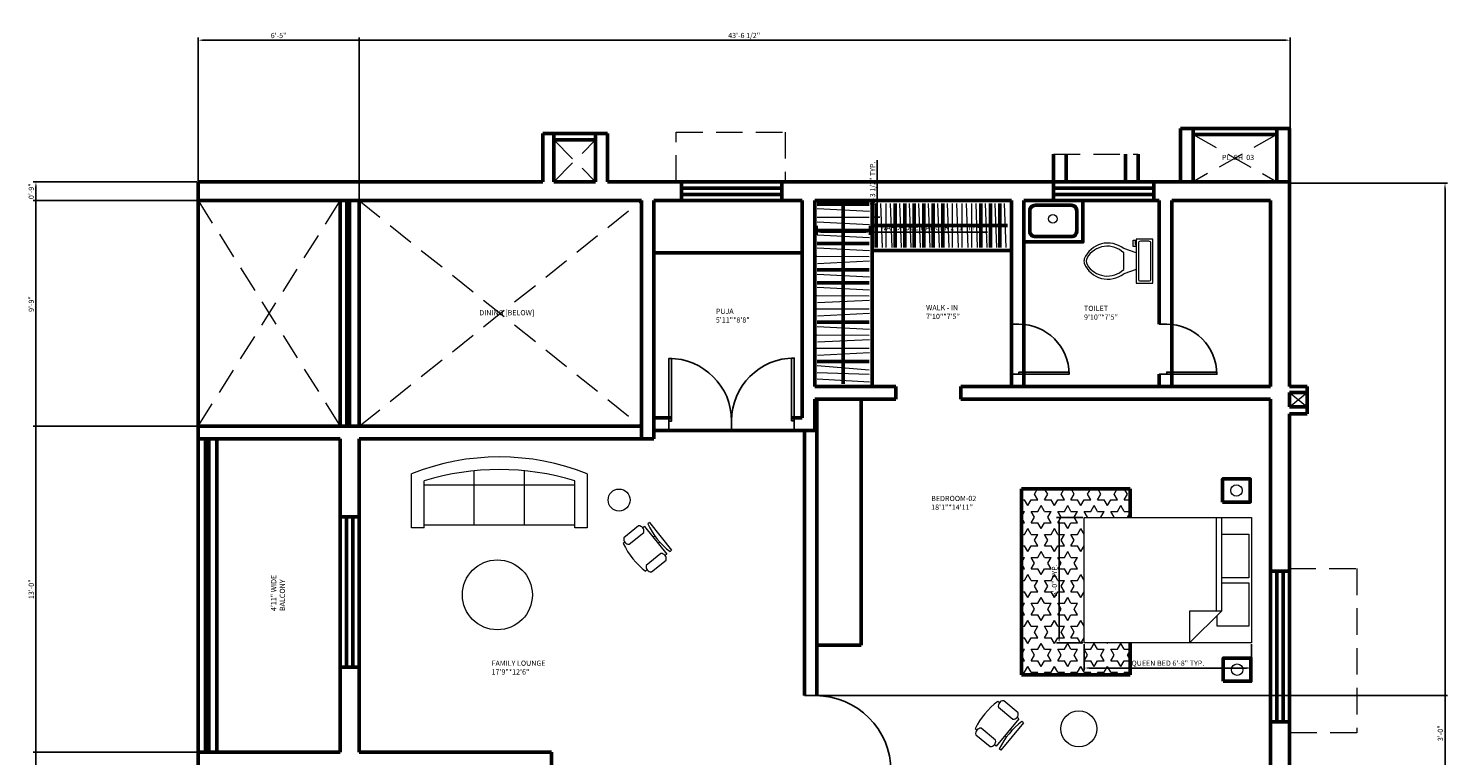
# Model space of a CAD drawing. Units: inches. Extents: x 5312 to 23584, y 2846 to 7447.
# Tile 6 of 12: x 9893 to 10572, y 3551 to 3899. Entities that reach past the tile are written whole.
import ezdxf

# ---------------------------------------------------------------- set-up
doc = ezdxf.new("R2010")
doc.units = ezdxf.units.IN
doc.linetypes.add('DASHED', pattern=[19.05, 12.7, -6.35])
for name, color, linetype, lineweight in [('A-ANNO-DIMS', 2, 'Continuous', 18), ('A-ANNO-TEXT', 3, 'Continuous', 18), ('A-AREA-IDEN', 7, 'Continuous', 18), ('A-DOOR', 4, 'Continuous', 25), ('A-FLOR-FIXT', 9, 'Continuous', 18), ('A-FLOR-OVHD', 8, 'DASHED', 18), ('A-FLOR-PATT', 252, 'Continuous', 13), ('A-FURN', 8, 'Continuous', 18), ('A-WALL', 7, 'Continuous', 50)]:
    doc.layers.add(name, color=color, linetype=linetype, lineweight=lineweight)
doc.styles.get("Standard").update_dxf_attribs({"font": 'arial.ttf'})
doc.dimstyles.new('ISO-25', dxfattribs={"dimtxt": 2.5, "dimasz": 2.5, "dimexe": 1.25, "dimexo": 0.625, "dimtad": 1, "dimlunit": 3, "dimtxsty": 'Standard', "dimcen": 2.5, "dimadec": 0, "dimazin": 0, "dimtfac": 1, "dimtmove": 0, "dimatfit": 3, "dimfxl": 1, "dimarcsym": 0})

# ---------------------------------------------------------------- blocks, each defined once
blk = doc.blocks.new('*U2')
for p, q in [((0, 0), (0, -6)), ((40, 0), (40, -6))]:
    blk.add_line(p, q)
blk.add_lwpolyline([(0, 0), (0, 40), (1.75, 40), (1.75, 0)], close=True)
blk.add_arc((0, 0), 40, 0, 90)
blk = doc.blocks.new('Sofa - Roundback 7 ft.')
for p, q in [((-12.00002, -32.4421), (-12.00003, -6.5971)), ((11.99997, -32.4421), (11.99998, -6.5971)), ((-36.000027, -34), (-36.000027, -11.4696)), ((-35.999844, -13.3819), (35.9998, -13.3819)), ((35.99998, -34), (35.99998, -11.4696)), ((-36.000027, -32.4421), (35.99998, -32.4421))]:
    blk.add_line(p, q)
for points in [[(-36.000027, -34), (-42.000027, -34), (-42.000027, -8)], [(41.99998, -8), (41.99998, -34), (35.99998, -34)]]:
    blk.add_lwpolyline(points)
for centre, radius, start, end in [((0, -114.25), 114.25, 68.43141, 111.5686), ((-0.00001, -127.1968), 121.1968, 72.72033, 107.2797)]:
    blk.add_arc(centre, radius, start, end)
blk = doc.blocks.new('Chair - Desk')
for p, q in [((-8.5, 0), (-8.5, -1)), ((-8.5, 0), (8.5, 0)), ((8.5, 0), (8.5, -1)), ((-10.5, -5), (-10.5, -14)), ((-8.5, -3), (-8.5, -4)), ((-8.5, -3), (8.5, -3)), ((-6.5, -14), (-6.5, -5)), ((-2, -3), (-2, -1.9355)), ((2, -1.9576), (2, -3)), ((6.5, -5), (6.5, -14)), ((8.5, -3), (8.5, -4)), ((10.5, -14), (10.5, -5)), ((-8.5, -15), (-8.5, -16)), ((8.5, -15), (8.5, -16))]:
    blk.add_line(p, q)
for centre, radius, start, end in [((-8.5, -6.5), 2.5, 36.8699, 143.1301), ((0, 34.625), 36.625, 256.5803, 283.4197), ((8.5, -6.5), 2.5, 36.8699, 143.1301), ((-8.5, -12.5), 2.5, 216.8699, 323.1301), ((0, 19.625), 36.625, 256.5803, 283.4197), ((8.5, -12.5), 2.5, 216.8699, 323.1301)]:
    blk.add_arc(centre, radius, start, end)
blk = doc.blocks.new('Toilet - top')
for p, q in [((9.5, -6), (9.5, -2)), ((-10, -8.5), (-8, -8.5)), ((-10, -9.5), (-10, -8.5)), ((-7, -9.5), (-10, -9.5)), ((-8, -8.5), (-8, -8)), ((-7, -8), (-7, -9.5)), ((-4, -8), (-6, -14)), ((4, -8), (6, -14)), ((4, -14), (-4, -14))]:
    blk.add_line(p, q)
blk.add_lwpolyline([(10.5, -8), (10.5, 0), (-10.5, 0), (-10.5, -8)], close=True)
for points in [[(-9.5, -2), (-9.5, -6)], [(8.5, -1), (-8.5, -1)], [(-8.5, -7), (8.5, -7)]]:
    blk.add_lwpolyline(points)
for centre, radius, start, end in [((-8.62, -1.88), 0.884, 81.8699, 188.1301), ((-8.62, -6.12), 0.884, 171.8699, 278.1301), ((8.62, -1.88), 0.884, 351.8699, 98.1301), ((8.62, -6.12), 0.884, 261.8699, 8.1301), ((3.52, -21.58), 12.17, 141.46911, 247.97143), ((4.2, -21.82), 11.33, 136.36773, 238.94682), ((-3.52, -21.58), 12.17, 292.02843, 38.53071), ((-4.2, -21.82), 11.33, 301.05301, 43.63209), ((0, -27.88), 4, 245.73182, 294.26817), ((0, -29), 4, 254.86053, 285.13947)]:
    blk.add_arc(centre, radius, start, end)
blk = doc.blocks.new('Bed - Queen')
for p, q in [((0, -80.00003), (0, 0)), ((0, 0), (59.99999, 0)), ((59.99999, 0), (59.99999, -80.00003)), ((7.99999, -1.2), (28.79998, -1.2)), ((7.99999, -14.4), (7.99999, -1.2)), ((28.79998, -1.2), (28.79998, -14.4)), ((31.19999, -1.2), (51.99999, -1.2)), ((31.19999, -14.4), (31.19999, -1.2)), ((51.99999, -1.2), (51.99999, -16.4)), ((0, -14.4), (44.8, -14.4)), ((44.8, -16.8), (0, -16.8)), ((59.99999, -29.6), (44.8, -14.4)), ((44.8, -14.4), (44.8, -29.6)), ((51.99999, -16.4), (46.79936, -16.4)), ((44.8, -29.6), (59.99999, -29.6)), ((59.99999, -80.00003), (0, -80.00003))]:
    blk.add_line(p, q)
blk = doc.blocks.new('WARDROBE-HANGER')
for p, q in [((0, 3.4), (24.8, 3.4)), ((0, 1.32), (24.99, 0))]:
    blk.add_line(p, q)
blk = doc.blocks.new('WARDROBE-HANGER-B')
for p, q in [((0, 21.08), (0.79, 0)), ((2.48, 21.08), (2.48, 0))]:
    blk.add_line(p, q)
blk = doc.blocks.new('*D25')
at = {"layer": 'A-ANNO-DIMS', "color": 0, "lineweight": -2, "transparency": 16777216}
for p, q in [((10398.36, 3604.72), (10398.36, 3592.09)), ((10478.36, 3604.72), (10478.36, 3592.09)), ((10400.86, 3593.34), (10475.86, 3593.34))]:
    blk.add_line(p, q, dxfattribs=at)
at = {"layer": 'A-ANNO-DIMS', "color": 0, "transparency": 16777216}
for points in [[(10400.86, 3593.76), (10400.86, 3592.92), (10398.36, 3593.34)], [(10475.86, 3593.76), (10475.86, 3592.92), (10478.36, 3593.34)]]:
    blk.add_solid(points, dxfattribs=at)
at = {"layer": 'DEFPOINTS', "color": 0, "transparency": 16777216}
for p in [(10398.36, 3605.34), (10478.36, 3605.34), (10478.36, 3593.34)]:
    blk.add_point(p, dxfattribs=at)
at = {"layer": 'A-ANNO-DIMS', "color": 0, "transparency": 16777216, "insert": (10438.36, 3595.33), "char_height": 2.5, "attachment_point": 5}
blk.add_mtext('QUEEN BED 6\'-8" TYP.', dxfattribs=at)
blk = doc.blocks.new('*D26')
at = {"layer": 'A-ANNO-DIMS', "color": 0, "lineweight": -2, "transparency": 16777216}
for p, q in [((10397.74, 3665.34), (10385.11, 3665.34)), ((10386.36, 3662.84), (10386.36, 3607.84)), ((10397.74, 3605.34), (10385.11, 3605.34))]:
    blk.add_line(p, q, dxfattribs=at)
at = {"layer": 'A-ANNO-DIMS', "color": 0, "transparency": 16777216}
for points in [[(10385.95, 3662.84), (10386.78, 3662.84), (10386.36, 3665.34)], [(10385.95, 3607.84), (10386.78, 3607.84), (10386.36, 3605.34)]]:
    blk.add_solid(points, dxfattribs=at)
at = {"layer": 'DEFPOINTS', "color": 0, "transparency": 16777216}
for p in [(10398.36, 3665.34), (10386.36, 3605.34), (10398.36, 3605.34)]:
    blk.add_point(p, dxfattribs=at)
at = {"layer": 'A-ANNO-DIMS', "color": 0, "transparency": 16777216, "insert": (10384.46, 3635.34), "char_height": 2.5, "attachment_point": 5, "rotation": 90}
blk.add_mtext('5\'-0" TYP.', dxfattribs=at)
blk = doc.blocks.new('*D35')
at = {"layer": 'A-ANNO-DIMS', "color": 0, "lineweight": -2, "transparency": 16777216}
for p, q in [((10270.63, 3805.02), (10270.63, 3800.65)), ((10273.13, 3801.9), (10293.12, 3801.9)), ((10295.62, 3805.02), (10295.62, 3800.65)), ((10295.62, 3801.9), (10352.16, 3801.9))]:
    blk.add_line(p, q, dxfattribs=at)
at = {"layer": 'A-ANNO-DIMS', "color": 0, "transparency": 16777216}
for points in [[(10273.13, 3802.31), (10273.13, 3801.48), (10270.63, 3801.9)], [(10293.12, 3802.31), (10293.12, 3801.48), (10295.62, 3801.9)]]:
    blk.add_solid(points, dxfattribs=at)
at = {"layer": 'DEFPOINTS', "color": 0, "transparency": 16777216}
for p in [(10270.63, 3805.65), (10295.62, 3805.65), (10295.62, 3801.9)]:
    blk.add_point(p, dxfattribs=at)
at = {"layer": 'A-ANNO-DIMS', "color": 0, "transparency": 16777216, "insert": (10325.14, 3803.82), "char_height": 2.5, "attachment_point": 5}
blk.add_mtext('WARDROBE HANGER 2\'-1" TYP.', dxfattribs=at)
blk = doc.blocks.new('*D36')
at = {"layer": 'A-ANNO-DIMS', "color": 0, "lineweight": -2, "transparency": 16777216}
for p, q in [((10299.37, 3811.55), (10299.37, 3836.36)), ((10296.25, 3809.05), (10300.62, 3809.05)), ((10299.37, 3805.65), (10299.37, 3809.05)), ((10296.25, 3805.65), (10300.62, 3805.65)), ((10299.37, 3803.15), (10299.37, 3800.65))]:
    blk.add_line(p, q, dxfattribs=at)
at = {"layer": 'A-ANNO-DIMS', "color": 0, "transparency": 16777216}
for points in [[(10298.95, 3811.55), (10299.79, 3811.55), (10299.37, 3809.05)], [(10298.95, 3803.15), (10299.79, 3803.15), (10299.37, 3805.65)]]:
    blk.add_solid(points, dxfattribs=at)
at = {"layer": 'DEFPOINTS', "color": 0, "transparency": 16777216}
for p in [(10295.62, 3809.05), (10299.37, 3809.05), (10295.62, 3805.65)]:
    blk.add_point(p, dxfattribs=at)
at = {"layer": 'A-ANNO-DIMS', "color": 0, "transparency": 16777216, "insert": (10297.45, 3825.21), "char_height": 2.5, "attachment_point": 5, "rotation": 90}
blk.add_mtext('0\'-3 1/2" TYP.', dxfattribs=at)
blk = doc.blocks.new('*D71')
at = {"layer": 'A-ANNO-DIMS', "color": 0, "lineweight": -2, "transparency": 16777216}
for p, q in [((9974.51, 3826.67), (9974.51, 3895.08)), ((9977.01, 3893.83), (10494.36, 3893.83)), ((10496.86, 3826), (10496.86, 3895.08))]:
    blk.add_line(p, q, dxfattribs=at)
at = {"layer": 'A-ANNO-DIMS', "color": 0, "transparency": 16777216}
for points in [[(9977.01, 3894.25), (9977.01, 3893.42), (9974.51, 3893.83)], [(10494.36, 3894.25), (10494.36, 3893.42), (10496.86, 3893.83)]]:
    blk.add_solid(points, dxfattribs=at)
at = {"layer": 'DEFPOINTS', "color": 0, "transparency": 16777216}
for p in [(10496.86, 3893.83), (9974.51, 3826.04), (10496.86, 3825.38)]:
    blk.add_point(p, dxfattribs=at)
at = {"layer": 'A-ANNO-DIMS', "color": 0, "transparency": 16777216, "insert": (10235.69, 3895.75), "char_height": 2.5, "attachment_point": 5}
blk.add_mtext('43\'-6 1/2"', dxfattribs=at)
blk = doc.blocks.new('*D72')
at = {"layer": 'A-ANNO-DIMS', "color": 0, "lineweight": -2, "transparency": 16777216}
for p, q in [((10497.49, 3825.38), (10572.19, 3825.38)), ((10570.94, 3822.88), (10570.94, 3090.84)), ((10497.14, 3088.34), (10572.19, 3088.34))]:
    blk.add_line(p, q, dxfattribs=at)
at = {"layer": 'A-ANNO-DIMS', "color": 0, "transparency": 16777216}
for points in [[(10570.52, 3822.88), (10571.35, 3822.88), (10570.94, 3825.38)], [(10570.52, 3090.84), (10571.35, 3090.84), (10570.94, 3088.34)]]:
    blk.add_solid(points, dxfattribs=at)
at = {"layer": 'DEFPOINTS', "color": 0, "transparency": 16777216}
for p in [(10496.86, 3825.38), (10496.51, 3088.34), (10570.94, 3088.34)]:
    blk.add_point(p, dxfattribs=at)
at = {"layer": 'A-ANNO-DIMS', "color": 0, "transparency": 16777216, "insert": (10569.03, 3456.86), "char_height": 2.5, "attachment_point": 5, "rotation": 90}
blk.add_mtext('61\'-5"', dxfattribs=at)
blk = doc.blocks.new('*D73')
at = {"layer": 'A-ANNO-DIMS', "color": 0, "lineweight": -2, "transparency": 16777216}
for p, q in [((9973.89, 3826.04), (9895.66, 3826.04)), ((9896.91, 3823.54), (9896.91, 3127.54)), ((9973.89, 3125.04), (9895.66, 3125.04))]:
    blk.add_line(p, q, dxfattribs=at)
at = {"layer": 'A-ANNO-DIMS', "color": 0, "transparency": 16777216}
for points in [[(9896.49, 3823.54), (9897.32, 3823.54), (9896.91, 3826.04)], [(9896.49, 3127.54), (9897.32, 3127.54), (9896.91, 3125.04)]]:
    blk.add_solid(points, dxfattribs=at)
at = {"layer": 'DEFPOINTS', "color": 0, "transparency": 16777216}
for p in [(9974.51, 3826.04), (9896.91, 3125.04), (9974.51, 3125.04)]:
    blk.add_point(p, dxfattribs=at)
at = {"layer": 'A-ANNO-DIMS', "color": 0, "transparency": 16777216, "insert": (9895.01, 3475.54), "char_height": 2.5, "attachment_point": 5, "rotation": 90}
blk.add_mtext('58\'-5"', dxfattribs=at)
blk = doc.blocks.new('*D74')
at = {"layer": 'A-ANNO-DIMS', "color": 0, "lineweight": -2, "transparency": 16777216}
for p, q in [((9974.51, 3709.67), (9974.51, 3895.08)), ((9977.01, 3893.83), (10049.01, 3893.83)), ((10051.51, 3709.67), (10051.51, 3895.08))]:
    blk.add_line(p, q, dxfattribs=at)
at = {"layer": 'A-ANNO-DIMS', "color": 0, "transparency": 16777216}
for points in [[(9977.01, 3894.25), (9977.01, 3893.42), (9974.51, 3893.83)], [(10049.01, 3894.25), (10049.01, 3893.42), (10051.51, 3893.83)]]:
    blk.add_solid(points, dxfattribs=at)
at = {"layer": 'DEFPOINTS', "color": 0, "transparency": 16777216}
for p in [(10051.51, 3893.83), (9974.51, 3709.04), (10051.51, 3709.04)]:
    blk.add_point(p, dxfattribs=at)
at = {"layer": 'A-ANNO-DIMS', "color": 0, "transparency": 16777216, "insert": (10013.01, 3895.74), "char_height": 2.5, "attachment_point": 5}
blk.add_mtext('6\'-5"', dxfattribs=at)
blk = doc.blocks.new('*D75')
at = {"layer": 'A-ANNO-DIMS', "color": 0, "lineweight": -2, "transparency": 16777216}
for p, q in [((9973.89, 3826.04), (9895.66, 3826.04)), ((9896.91, 3823.54), (9896.91, 3711.54)), ((9973.89, 3709.04), (9895.66, 3709.04))]:
    blk.add_line(p, q, dxfattribs=at)
at = {"layer": 'A-ANNO-DIMS', "color": 0, "transparency": 16777216}
for points in [[(9896.49, 3823.54), (9897.32, 3823.54), (9896.91, 3826.04)], [(9896.49, 3711.54), (9897.32, 3711.54), (9896.91, 3709.04)]]:
    blk.add_solid(points, dxfattribs=at)
at = {"layer": 'DEFPOINTS', "color": 0, "transparency": 16777216}
for p in [(9974.51, 3826.04), (9896.91, 3709.04), (9974.51, 3709.04)]:
    blk.add_point(p, dxfattribs=at)
at = {"layer": 'A-ANNO-DIMS', "color": 0, "transparency": 16777216, "insert": (9895.01, 3767.54), "char_height": 2.5, "attachment_point": 5, "rotation": 90}
blk.add_mtext('9\'-9"', dxfattribs=at)
blk = doc.blocks.new('*D76')
at = {"layer": 'A-ANNO-DIMS', "color": 0, "lineweight": -2, "transparency": 16777216}
for p, q in [((9973.89, 3709.04), (9895.66, 3709.04)), ((9896.91, 3706.54), (9896.91, 3555.54)), ((9973.89, 3553.04), (9895.66, 3553.04))]:
    blk.add_line(p, q, dxfattribs=at)
at = {"layer": 'A-ANNO-DIMS', "color": 0, "transparency": 16777216}
for points in [[(9896.49, 3706.54), (9897.32, 3706.54), (9896.91, 3709.04)], [(9896.49, 3555.54), (9897.32, 3555.54), (9896.91, 3553.04)]]:
    blk.add_solid(points, dxfattribs=at)
at = {"layer": 'DEFPOINTS', "color": 0, "transparency": 16777216}
for p in [(9974.51, 3709.04), (9896.91, 3553.04), (9974.51, 3553.04)]:
    blk.add_point(p, dxfattribs=at)
at = {"layer": 'A-ANNO-DIMS', "color": 0, "transparency": 16777216, "insert": (9895.01, 3631.04), "char_height": 2.5, "attachment_point": 5, "rotation": 90}
blk.add_mtext('13\'-0"', dxfattribs=at)
blk = doc.blocks.new('*D77')
at = {"layer": 'A-ANNO-DIMS', "color": 0, "lineweight": -2, "transparency": 16777216}
for p, q in [((9973.89, 3553.04), (9895.66, 3553.04)), ((9896.91, 3550.54), (9896.91, 3388.54)), ((9982.89, 3386.04), (9895.66, 3386.04))]:
    blk.add_line(p, q, dxfattribs=at)
at = {"layer": 'A-ANNO-DIMS', "color": 0, "transparency": 16777216}
for points in [[(9896.49, 3550.54), (9897.32, 3550.54), (9896.91, 3553.04)], [(9896.49, 3388.54), (9897.32, 3388.54), (9896.91, 3386.04)]]:
    blk.add_solid(points, dxfattribs=at)
at = {"layer": 'DEFPOINTS', "color": 0, "transparency": 16777216}
for p in [(9974.51, 3553.04), (9896.91, 3386.04), (9983.51, 3386.04)]:
    blk.add_point(p, dxfattribs=at)
at = {"layer": 'A-ANNO-DIMS', "color": 0, "transparency": 16777216, "insert": (9895.01, 3469.54), "char_height": 2.5, "attachment_point": 5, "rotation": 90}
blk.add_mtext('13\'-11"', dxfattribs=at)
blk = doc.blocks.new('*D80')
at = {"layer": 'A-ANNO-DIMS', "color": 0, "lineweight": -2, "transparency": 16777216}
for p, q in [((9973.89, 3826.04), (9895.66, 3826.04)), ((9896.91, 3823.54), (9896.91, 3819.54)), ((9973.89, 3817.04), (9895.66, 3817.04))]:
    blk.add_line(p, q, dxfattribs=at)
at = {"layer": 'A-ANNO-DIMS', "color": 0, "transparency": 16777216}
for points in [[(9896.49, 3823.54), (9897.32, 3823.54), (9896.91, 3826.04)], [(9896.49, 3819.54), (9897.32, 3819.54), (9896.91, 3817.04)]]:
    blk.add_solid(points, dxfattribs=at)
at = {"layer": 'DEFPOINTS', "color": 0, "transparency": 16777216}
for p in [(9974.51, 3826.04), (9896.91, 3817.04), (9974.51, 3817.04)]:
    blk.add_point(p, dxfattribs=at)
at = {"layer": 'A-ANNO-DIMS', "color": 0, "transparency": 16777216, "insert": (9895.01, 3821.54), "char_height": 2.5, "attachment_point": 5, "rotation": 90}
blk.add_mtext('0\'-9"', dxfattribs=at)
blk = doc.blocks.new('*D82')
at = {"layer": 'A-ANNO-DIMS', "color": 0, "lineweight": -2, "transparency": 16777216}
for p, q in [((10265.14, 3580.12), (10572.19, 3580.12)), ((10570.94, 3577.62), (10570.94, 3546.62)), ((10265.14, 3544.12), (10572.19, 3544.12))]:
    blk.add_line(p, q, dxfattribs=at)
at = {"layer": 'A-ANNO-DIMS', "color": 0, "transparency": 16777216}
for points in [[(10570.52, 3577.62), (10571.35, 3577.62), (10570.94, 3580.12)], [(10570.52, 3546.62), (10571.35, 3546.62), (10570.94, 3544.12)]]:
    blk.add_solid(points, dxfattribs=at)
at = {"layer": 'DEFPOINTS', "color": 0, "transparency": 16777216}
for p in [(10264.51, 3580.12), (10264.51, 3544.12), (10570.94, 3544.12)]:
    blk.add_point(p, dxfattribs=at)
at = {"layer": 'A-ANNO-DIMS', "color": 0, "transparency": 16777216, "insert": (10569.03, 3562.12), "char_height": 2.5, "attachment_point": 5, "rotation": 90}
blk.add_mtext('3\'-0"', dxfattribs=at)

msp = doc.modelspace()

# ---------------------------------------------------------------- hatches: boundary and pattern name
at = {"layer": 'A-FLOR-PATT'}
h = msp.add_hatch(dxfattribs=at)
h.set_pattern_fill('STARS', color=256)
h.set_pattern_definition([(0, (143.128, -197.685), (0, 5.4992613), [3.175, -3.175]), (60, (143.128, -197.685), (-4.7625, 2.7496307), [3.175, -3.175]), (120, (144.716, -194.935), (-4.7625, -2.7496307), [3.175, -3.175])])
h.paths.add_polyline_path([(10398.363, 3665.341), (10420.302, 3665.341), (10420.302, 3679.171), (10368.287, 3679.171), (10368.287, 3590.007), (10420.302, 3590.007), (10420.302, 3605.341), (10398.363, 3605.341)])

# ---------------------------------------------------------------- linework, layer by layer
at = {"layer": 'A-FLOR-OVHD'}
for p, q in [((10203.179, 3826.044), (10203.179, 3849.843)), ((10203.179, 3849.843), (10255.248, 3849.843)), ((10255.248, 3849.843), (10255.248, 3826.044)), ((10144.712, 3846.108), (10144.712, 3846.108)), ((10144.712, 3846.108), (10164.599, 3826.044)), ((10144.712, 3826.044), (10164.599, 3846.108)), ((10450.49, 3848.735), (10490.514, 3826.044)), ((10490.514, 3848.735), (10450.49, 3826.044)), ((10383.677, 3839.224), (10424.112, 3839.224)), ((9974.514, 3817.044), (10042.514, 3709.044)), ((9974.514, 3709.044), (10042.514, 3817.044)), ((10051.514, 3817.044), (10186.514, 3709.044)), ((10051.514, 3709.044), (10186.514, 3817.044)), ((10496.514, 3725.243), (10504.951, 3718.3)), ((10496.514, 3718.3), (10504.951, 3725.243)), ((10496.514, 3640.969), (10528.686, 3640.969)), ((10528.686, 3640.969), (10528.686, 3562.391)), ((10528.686, 3562.391), (10496.514, 3562.391))]:
    msp.add_line(p, q, dxfattribs=at)
at = {"layer": 'A-FURN'}
for p, q in [((10305.486, 3815.641), (10306.276, 3794.559)), ((10310.036, 3815.641), (10310.826, 3794.559)), ((10314.586, 3815.641), (10315.376, 3794.559)), ((10319.136, 3815.641), (10319.926, 3794.559)), ((10323.686, 3815.641), (10324.476, 3794.559)), ((10328.235, 3815.641), (10329.025, 3794.559)), ((10346.435, 3815.641), (10347.225, 3794.559)), ((10350.985, 3815.641), (10351.775, 3794.559)), ((10355.535, 3815.641), (10356.325, 3794.559)), ((10360.085, 3815.641), (10360.875, 3794.559)), ((10270.629, 3813.242), (10295.62, 3811.92)), ((10270.629, 3800.697), (10295.62, 3799.374)), ((10270.629, 3794.424), (10295.62, 3793.102)), ((10270.629, 3781.879), (10295.62, 3780.556)), ((10270.629, 3775.606), (10295.62, 3774.284)), ((10270.629, 3756.788), (10295.62, 3755.465)), ((10270.629, 3731.697), (10295.62, 3730.375))]:
    msp.add_line(p, q, dxfattribs=at)
for centre, radius in [((10383.307, 3808.29), 2.047), ((10471.157, 3678.295), 2.744), ((10175.876, 3673.737), 5.262), ((10117.642, 3628.36), 16.727), ((10471.504, 3592.534), 2.744), ((10395.741, 3564.219), 8.619)]:
    msp.add_circle(centre, radius, dxfattribs=at)
at = {"layer": 'A-WALL'}
for p, q in [((10496.514, 3851.585), (10444.49, 3851.585)), ((10444.49, 3851.585), (10444.49, 3826.044)), ((10450.49, 3851.585), (10450.49, 3826.044)), ((10490.514, 3826.044), (10490.514, 3851.585)), ((10496.514, 3826.044), (10496.514, 3851.585)), ((10139.398, 3846.108), (10139.398, 3849.106)), ((10139.398, 3849.106), (10170.255, 3849.106)), ((10139.398, 3846.108), (10139.398, 3826.044)), ((10144.712, 3849.106), (10144.712, 3826.044)), ((10164.33, 3846.108), (10144.712, 3846.108)), ((10164.599, 3846.108), (10164.33, 3846.108)), ((10164.599, 3849.106), (10164.599, 3826.044)), ((10170.255, 3849.106), (10170.255, 3846.108)), ((10170.255, 3826.044), (10170.255, 3846.108)), ((10450.49, 3848.735), (10490.514, 3848.735)), ((10383.677, 3826.044), (10383.677, 3839.224)), ((10389.677, 3826.044), (10389.677, 3839.224)), ((10418.112, 3826.044), (10418.112, 3839.224)), ((10424.112, 3839.224), (10424.112, 3838.603)), ((10424.112, 3826.044), (10424.112, 3838.603)), ((9974.514, 3826.044), (9974.514, 3125.044)), ((9974.514, 3826.044), (10139.398, 3826.044)), ((10144.712, 3826.044), (10164.599, 3826.044)), ((10170.255, 3826.044), (10170.255, 3826.044)), ((10170.255, 3826.044), (10496.514, 3826.044)), ((10205.784, 3826.044), (10253.784, 3826.044)), ((10205.784, 3817.044), (10205.784, 3826.044)), ((10205.784, 3823.044), (10253.784, 3823.044)), ((10253.784, 3826.044), (10253.784, 3817.044)), ((10383.677, 3826.044), (10431.677, 3826.044)), ((10383.677, 3817.044), (10383.677, 3826.044)), ((10383.677, 3823.044), (10431.677, 3823.044)), ((10431.677, 3826.044), (10431.677, 3817.044)), ((10496.514, 3826.044), (10496.514, 3728.044)), ((10496.514, 3826.044), (10496.862, 3825.376)), ((9974.514, 3817.044), (10186.514, 3817.044)), ((10042.514, 3817.044), (10042.514, 3709.044)), ((10045.614, 3817.044), (10045.614, 3709.044)), ((10046.923, 3817.044), (10046.923, 3709.044)), ((10051.514, 3817.044), (10051.514, 3709.044)), ((10186.514, 3817.044), (10186.514, 3703.044)), ((10192.514, 3817.044), (10192.514, 3703.044)), ((10192.514, 3817.044), (10263.514, 3817.044)), ((10253.784, 3820.044), (10205.784, 3820.044)), ((10253.784, 3817.044), (10205.784, 3817.044)), ((10263.514, 3817.044), (10263.514, 3713.044)), ((10269.514, 3817.044), (10269.514, 3728.044)), ((10269.514, 3817.044), (10363.514, 3817.044)), ((10283.03, 3816.362), (10283.03, 3729.279)), ((10296.889, 3728.044), (10296.889, 3817.044)), ((10298.863, 3815.641), (10298.863, 3794.559)), ((10307.963, 3815.641), (10307.963, 3794.559)), ((10312.513, 3815.641), (10312.513, 3794.559)), ((10317.063, 3815.641), (10317.063, 3794.559)), ((10321.612, 3815.641), (10321.612, 3794.559)), ((10326.162, 3815.641), (10326.162, 3794.559)), ((10330.712, 3815.641), (10330.712, 3794.559)), ((10348.912, 3815.641), (10348.912, 3794.559)), ((10353.462, 3815.641), (10353.462, 3794.559)), ((10358.011, 3815.641), (10358.011, 3794.559)), ((10363.514, 3817.044), (10363.514, 3728.044)), ((10369.514, 3817.044), (10369.514, 3728.044)), ((10369.514, 3817.044), (10434.209, 3817.044)), ((10431.677, 3820.044), (10383.677, 3820.044)), ((10431.677, 3817.044), (10383.677, 3817.044)), ((10434.209, 3817.044), (10434.209, 3757.917)), ((10440.209, 3817.044), (10440.209, 3728.044)), ((10440.209, 3817.044), (10487.514, 3817.044)), ((10487.514, 3817.044), (10487.514, 3728.044)), ((10270.629, 3815.321), (10295.431, 3815.321)), ((10270.629, 3802.775), (10295.431, 3802.775)), ((10297.733, 3805.079), (10361.591, 3805.079)), ((10270.629, 3796.503), (10295.431, 3796.503)), ((10192.514, 3791.992), (10263.514, 3791.992)), ((10296.889, 3793.154), (10363.514, 3793.154)), ((10270.629, 3783.957), (10295.431, 3783.957)), ((10270.629, 3777.684), (10295.431, 3777.684)), ((10270.629, 3758.866), (10295.431, 3758.866)), ((10270.629, 3740.048), (10295.431, 3740.048)), ((10434.209, 3733.917), (10434.209, 3728.044)), ((10269.514, 3728.044), (10308.169, 3728.044)), ((10308.169, 3728.044), (10308.169, 3722.044)), ((10339.283, 3728.044), (10339.283, 3722.044)), ((10339.283, 3728.044), (10369.514, 3728.044)), ((10369.514, 3728.044), (10487.514, 3728.044)), ((10496.514, 3728.044), (10504.951, 3728.044)), ((10504.951, 3728.044), (10504.951, 3725.243)), ((10269.514, 3722.044), (10308.169, 3722.044)), ((10269.514, 3722.044), (10269.514, 3707.044)), ((10270.514, 3722.044), (10270.514, 3580.113)), ((10291.661, 3722.044), (10291.661, 3604.353)), ((10339.283, 3722.044), (10487.514, 3722.044)), ((10487.514, 3722.044), (10487.514, 3464.044)), ((10504.951, 3725.243), (10496.514, 3725.243)), ((10496.514, 3725.243), (10496.514, 3718.3)), ((10504.951, 3725.243), (10504.951, 3718.3)), ((10496.514, 3718.3), (10504.951, 3718.3)), ((10504.951, 3715.012), (10496.514, 3715.012)), ((10496.514, 3715.012), (10496.514, 3500.066)), ((10504.951, 3718.3), (10504.951, 3715.012)), ((10186.514, 3709.044), (9974.514, 3709.044)), ((10192.514, 3713.044), (10200.996, 3713.044)), ((10192.514, 3707.044), (10269.514, 3707.044)), ((10229.646, 3713.044), (10229.714, 3713.044)), ((10258.371, 3713.044), (10263.514, 3713.044)), ((10264.514, 3707.044), (10264.514, 3580.118)), ((10042.514, 3703.044), (9974.514, 3703.044)), ((9978.025, 3703.044), (9978.025, 3553.044)), ((9979.604, 3703.044), (9979.604, 3553.044)), ((9983.514, 3703.044), (9983.514, 3553.044)), ((10042.514, 3703.044), (10042.514, 3553.044)), ((10192.514, 3703.044), (10051.514, 3703.044)), ((10051.514, 3703.044), (10051.514, 3553.044)), ((10420.302, 3679.171), (10368.287, 3679.171)), ((10368.287, 3679.171), (10368.287, 3590.007)), ((10420.302, 3665.341), (10420.302, 3679.171)), ((10042.514, 3593.75), (10042.514, 3665.75)), ((10042.514, 3665.75), (10051.514, 3665.75)), ((10045.514, 3593.75), (10045.514, 3665.75)), ((10048.514, 3665.75), (10048.514, 3593.75)), ((10051.514, 3665.75), (10051.514, 3593.75)), ((10487.514, 3567.629), (10487.514, 3639.629)), ((10487.514, 3639.629), (10496.514, 3639.629)), ((10490.514, 3567.629), (10490.514, 3639.629)), ((10493.514, 3639.629), (10493.514, 3567.629)), ((10496.514, 3639.629), (10496.514, 3567.629)), ((10420.302, 3605.341), (10420.302, 3590.007)), ((10291.661, 3604.353), (10270.514, 3604.353)), ((10051.514, 3593.75), (10042.514, 3593.75)), ((10420.302, 3590.007), (10368.287, 3590.007)), ((10496.514, 3567.629), (10487.514, 3567.629)), ((10042.514, 3553.044), (9974.514, 3553.044)), ((10143.514, 3553.044), (10051.514, 3553.044)), ((10143.514, 3553.044), (10143.514, 3544.747))]:
    msp.add_line(p, q, dxfattribs=at)
for points in [[(10369.514, 3817.044), (10397.694, 3817.044), (10397.694, 3797.315), (10369.514, 3797.315)], [(10464.529, 3672.753), (10477.785, 3672.753), (10477.785, 3683.836), (10464.529, 3683.836)], [(10464.876, 3586.993), (10478.132, 3586.993), (10478.132, 3598.075), (10464.876, 3598.075)]]:
    msp.add_lwpolyline(points, close=True, dxfattribs=at)
msp.add_lwpolyline([(10374.834, 3814.787), (10392.253, 3814.787, -0.4142136), (10394.753, 3812.287), (10394.753, 3802.33, -0.4142136), (10392.253, 3799.83), (10374.834, 3799.83, -0.4142136), (10372.334, 3802.33), (10372.334, 3812.287, -0.4142136)], format="xyb", close=True, dxfattribs=at)

# ---------------------------------------------------------------- block references
at = {"layer": 'A-DOOR', "rotation": 270}
for p, xscale, yscale, zscale in [((10367.114, 3733.917), -0.6, 0.6, 0.6), ((10437.809, 3733.917), -0.6, 0.6, 0.6), ((10269.914, 3544.118), -0.9, 0.9, 0.9)]:
    msp.add_blockref('*U2', p, dxfattribs=dict(at, xscale=xscale, yscale=yscale, zscale=zscale))
at = {"layer": 'A-DOOR', "yscale": 0.75, "zscale": 0.75}
for p, xscale in [((10199.684, 3711.544), 0.75), ((10259.684, 3711.694), -0.75)]:
    msp.add_blockref('*U2', p, dxfattribs=dict(at, xscale=xscale))
at = {"layer": 'A-FLOR-FIXT', "rotation": 270}
msp.add_blockref('Toilet - top', (10431.244, 3788.082), dxfattribs=at)
at = {"layer": 'A-FURN'}
for name, p in [('WARDROBE-HANGER-B', (10300.936, 3794.559)), ('WARDROBE-HANGER-B', (10332.785, 3794.559)), ('WARDROBE-HANGER-B', (10337.335, 3794.559)), ('WARDROBE-HANGER-B', (10341.885, 3794.559)), ('WARDROBE-HANGER', (10270.629, 3805.647)), ('Sofa - Roundback 7 ft.', (10118.617, 3694.361))]:
    msp.add_blockref(name, p, dxfattribs=at)
for name, p, rotation in [('WARDROBE-HANGER', (10295.406, 3791.522), 182.9188210945419), ('WARDROBE-HANGER', (10295.406, 3772.704), 182.9188210945419), ('WARDROBE-HANGER', (10295.406, 3766.432), 182.9188210945419), ('WARDROBE-HANGER', (10295.406, 3753.886), 182.9188210945419), ('WARDROBE-HANGER', (10295.406, 3747.614), 182.9188210945441), ('WARDROBE-HANGER', (10295.584, 3737.173), 178.1621402088064), ('Chair - Desk', (10195.67, 3656.337), 308.8980476431923), ('Bed - Queen', (10478.364, 3665.341), 270), ('Chair - Desk', (10363.936, 3560.624), 230.4373532912175)]:
    msp.add_blockref(name, p, dxfattribs=dict(at, rotation=rotation))

# ---------------------------------------------------------------- texts
at = {"layer": 'A-ANNO-TEXT', "char_height": 2.5, "attachment_point": 1}
for s, width, insert in [('PL  SH  03', 33.13848, (10464.28, 3838.949)), ('DINING [BELOW]', 70.29785, (10108.979, 3764.626))]:
    msp.add_mtext_dynamic_manual_height_columns(s, width=width, gutter_width=12.5, heights=[0], dxfattribs=dict(at, insert=insert))
at = {"layer": 'A-AREA-IDEN', "char_height": 2.5, "attachment_point": 1}
for s, width, insert in [('PUJA\\P5\'11"*8\'8"', 40.71834, (10222.15, 3765.333)), ('WALK - IN\\P7\'10"*7\'5"', 35.79404, (10322.708, 3767.043)), ('TOILET\\P9\'10"*7\'5"', 45.00296, (10398.258, 3766.703)), ('BEDROOM-02\\P18\'1"*14\'11"', 59.61937, (10325.153, 3675.748)), ('FAMILY LOUNGE\\P17\'9"*12\'6"', 71.33141, (10114.859, 3596.899))]:
    msp.add_mtext_dynamic_manual_height_columns(s, width=width, gutter_width=12.5, heights=[0], dxfattribs=dict(at, insert=insert))
at = {"layer": 'A-AREA-IDEN', "insert": (10009.385, 3620.602), "char_height": 2.5, "attachment_point": 1, "rotation": 90}
msp.add_mtext_dynamic_manual_height_columns('4\'11" WIDE \\PBALCONY', width=44.23368, gutter_width=12.5, heights=[0], dxfattribs=at)

# ---------------------------------------------------------------- dimensions: what is measured, and where the dimension line sits
at = {"layer": 'A-ANNO-DIMS'}
for base, p1, p2, picture, middle in [((10496.862, 3893.835), (9974.514, 3826.044), (10496.862, 3825.376), '*D71', (10235.688, 3895.753)), ((10051.514, 3893.835), (9974.514, 3709.044), (10051.514, 3709.044), '*D74', (10013.014, 3895.736))]:
    dim = msp.add_linear_dim(base=base, p1=p1, p2=p2, dimstyle='ISO-25', override={"dimdec": 1, "dimlfac": 1, "dimrnd": 0, "dimzin": 1, "dimdsep": 46, "dimlunit": 4, "dimfrac": 2}, dxfattribs=at)
    dim.commit()
    dim.dimension.update_dxf_attribs({"geometry": picture, "text_midpoint": middle})
for base, p1, p2, angle, picture, middle in [((10299.369, 3809.048), (10295.62, 3805.647), (10295.62, 3809.048), 90, '*D36', (10297.451, 3825.205)), ((10386.363, 3605.341), (10398.363, 3665.341), (10398.363, 3605.341), 270, '*D26', (10384.462, 3635.341))]:
    dim = msp.add_linear_dim(base=base, p1=p1, p2=p2, angle=angle, text='<> TYP.', dimstyle='ISO-25', override={"dimdec": 1, "dimrnd": 0, "dimzin": 1, "dimlunit": 4, "dimfrac": 2}, dxfattribs=at)
    dim.commit()
    dim.dimension.update_dxf_attribs({"geometry": picture, "text_midpoint": middle})
for base, p1, p2, picture, middle in [((9896.908, 3125.044), (9974.514, 3826.044), (9974.514, 3125.044), '*D73', (9895.007, 3475.544)), ((9896.908, 3709.044), (9974.514, 3826.044), (9974.514, 3709.044), '*D75', (9895.007, 3767.544)), ((9896.908, 3817.044), (9974.514, 3826.044), (9974.514, 3817.044), '*D80', (9895.007, 3821.544)), ((10570.936, 3088.341), (10496.862, 3825.376), (10496.514, 3088.341), '*D72', (10569.035, 3456.858)), ((9896.908, 3553.044), (9974.514, 3709.044), (9974.514, 3553.044), '*D76', (9895.006, 3631.044)), ((10570.936, 3544.118), (10264.514, 3580.118), (10264.514, 3544.118), '*D82', (10569.034, 3562.118)), ((9896.908, 3386.044), (9974.514, 3553.044), (9983.514, 3386.044), '*D77', (9895.006, 3469.544))]:
    dim = msp.add_linear_dim(base=base, p1=p1, p2=p2, angle=90, dimstyle='ISO-25', override={"dimdec": 1, "dimlfac": 1, "dimrnd": 0, "dimzin": 1, "dimdsep": 46, "dimlunit": 4, "dimfrac": 2}, dxfattribs=at)
    dim.commit()
    dim.dimension.update_dxf_attribs({"geometry": picture, "text_midpoint": middle})
for base, p1, p2, text, picture, middle in [((10295.62, 3801.898), (10270.629, 3805.647), (10295.62, 3805.647), 'WARDROBE HANGER <> TYP.', '*D35', (10325.141, 3803.817)), ((10478.364, 3593.341), (10398.363, 3605.341), (10478.364, 3605.341), 'QUEEN BED <> TYP.', '*D25', (10438.364, 3595.335))]:
    dim = msp.add_linear_dim(base=base, p1=p1, p2=p2, text=text, dimstyle='ISO-25', override={"dimdec": 1, "dimrnd": 0, "dimzin": 1, "dimlunit": 4, "dimfrac": 2}, dxfattribs=at)
    dim.commit()
    dim.dimension.update_dxf_attribs({"geometry": picture, "text_midpoint": middle})

doc.saveas('drawing.dxf')
